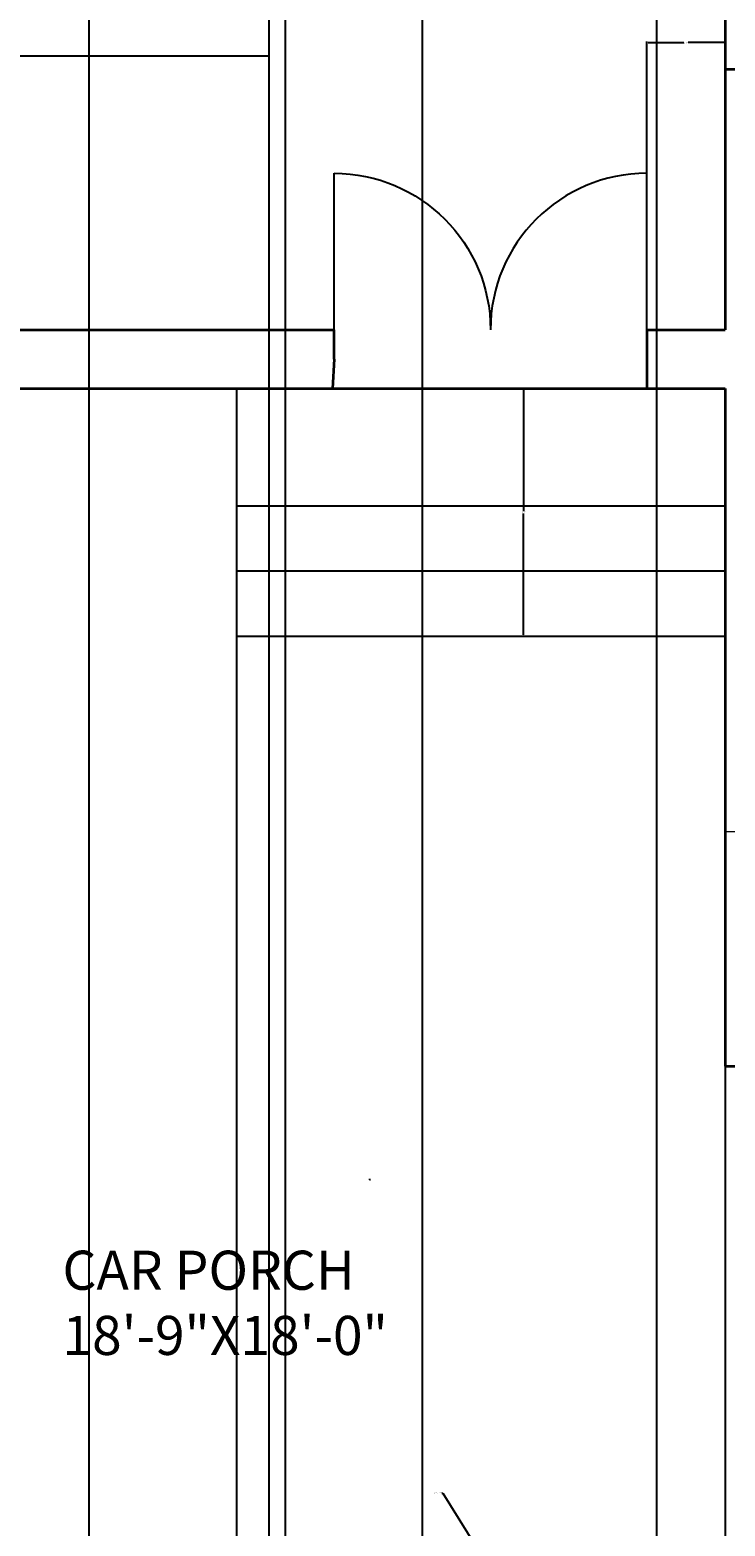
# Model space of a CAD drawing. Units: inches. Extents: x -10 to 502, y -868 to 56.
# Tile 7 of 14: x 165 to 272, y -724 to -495. Entities that reach past the tile are written whole.
import ezdxf

# ---------------------------------------------------------------- set-up
doc = ezdxf.new("R2010")
doc.units = ezdxf.units.IN
doc.header["$MEASUREMENT"] = 0
for name, color, linetype, lineweight in [('A-ANNO-DIMS', 2, 'Continuous', 18), ('A-AREA-IDEN', 7, 'Continuous', 18), ('A-DOOR', 4, 'Continuous', 25), ('A-FLOR-STRS', 7, 'Continuous', 25), ('A-GLAZ', 162, 'Continuous', 18), ('A-WALL', 7, 'Continuous', 35)]:
    doc.layers.add(name, color=color, linetype=linetype, lineweight=lineweight)
doc.styles.get("Standard").update_dxf_attribs({"font": 'arial.ttf'})
doc.dimstyles.get("Standard").update_dxf_attribs({"dimtxt": 0.18, "dimasz": 0.18, "dimexe": 0.18, "dimexo": 0.0625, "dimgap": 0.09, "dimtad": 0, "dimtih": 1, "dimtoh": 1, "dimdec": 0, "dimzin": 0, "dimdsep": 46, "dimlunit": 3, "dimtxsty": 'Standard', "dimcen": 0.09, "dimadec": 0, "dimazin": 0, "dimtfac": 1, "dimtdec": 0, "dimtofl": 0, "dimtmove": 0, "dimatfit": 3, "dimfxl": 1, "dimtolj": 1, "dimtzin": 0, "dimarcsym": 0})

# ---------------------------------------------------------------- blocks, each defined once
blk = doc.blocks.new('DOOR-SWING-24IN')
blk.add_line((24, 0), (24, 24))
blk.add_arc((24, 0), 24, 90, 180)
blk = doc.blocks.new('*D45')
at = {"layer": 'A-ANNO-DIMS', "color": 0, "lineweight": -2, "transparency": 16777216}
for p, q in [((196.98, -587.92), (196.98, -846.58)), ((271.95, -587.92), (271.95, -846.58)), ((197.16, -846.4), (234.14, -846.4)), ((271.77, -846.4), (234.8, -846.4))]:
    blk.add_line(p, q, dxfattribs=at)
at = {"layer": 'A-ANNO-DIMS', "color": 0, "transparency": 16777216}
for points in [[(197.16, -846.37), (197.16, -846.43), (196.98, -846.4)], [(271.77, -846.37), (271.77, -846.43), (271.95, -846.4)]]:
    blk.add_solid(points, dxfattribs=at)
at = {"layer": 'Defpoints', "color": 0, "transparency": 16777216}
for p in [(196.98, -587.85), (271.95, -587.85), (271.95, -846.4)]:
    blk.add_point(p, dxfattribs=at)
at = {"layer": 'A-ANNO-DIMS', "color": 0, "transparency": 16777216, "insert": (234.47, -846.4), "char_height": 0.18, "attachment_point": 5}
blk.add_mtext('\\A1;6\'-3"', dxfattribs=at)
blk = doc.blocks.new('*D46')
at = {"layer": 'A-ANNO-DIMS', "color": 0, "lineweight": -2, "transparency": 16777216}
for p, q in [((197.04, -549.85), (241.21, -549.85)), ((241.03, -550.03), (241.03, -568.67)), ((241.03, -587.67), (241.03, -569.03)), ((197.04, -587.85), (241.21, -587.85))]:
    blk.add_line(p, q, dxfattribs=at)
at = {"layer": 'A-ANNO-DIMS', "color": 0, "transparency": 16777216}
for points in [[(241, -550.03), (241.06, -550.03), (241.03, -549.85)], [(241, -587.67), (241.06, -587.67), (241.03, -587.85)]]:
    blk.add_solid(points, dxfattribs=at)
at = {"layer": 'Defpoints', "color": 0, "transparency": 16777216}
for p in [(196.98, -549.85), (196.98, -587.85), (241.03, -587.85)]:
    blk.add_point(p, dxfattribs=at)
at = {"layer": 'A-ANNO-DIMS', "color": 0, "transparency": 16777216, "insert": (241.03, -568.85), "char_height": 0.18, "attachment_point": 5}
blk.add_mtext('\\A1;3\'-2"', dxfattribs=at)
blk = doc.blocks.new('*D47')
at = {"layer": 'A-ANNO-DIMS', "color": 0, "lineweight": -2, "transparency": 16777216}
for p, q in [((91.95, -494.92), (91.95, -846.58)), ((201.95, -494.92), (201.95, -846.58)), ((92.13, -846.4), (146.62, -846.4)), ((201.77, -846.4), (147.28, -846.4))]:
    blk.add_line(p, q, dxfattribs=at)
at = {"layer": 'A-ANNO-DIMS', "color": 0, "transparency": 16777216}
for points in [[(92.13, -846.37), (92.13, -846.43), (91.95, -846.4)], [(201.77, -846.37), (201.77, -846.43), (201.95, -846.4)]]:
    blk.add_solid(points, dxfattribs=at)
at = {"layer": 'Defpoints', "color": 0, "transparency": 16777216}
for p in [(91.95, -494.85), (201.95, -494.85), (201.95, -846.4)]:
    blk.add_point(p, dxfattribs=at)
at = {"layer": 'A-ANNO-DIMS', "color": 0, "transparency": 16777216, "insert": (146.95, -846.4), "char_height": 0.18, "attachment_point": 5}
blk.add_mtext('\\A1;9\'-2"', dxfattribs=at)
blk = doc.blocks.new('*D53')
at = {"layer": 'A-ANNO-DIMS', "color": 0, "lineweight": -2, "transparency": 16777216}
for p, q in [((174.32, -443.06), (174.32, -846.58)), ((204.45, -443.92), (204.45, -846.58)), ((174.5, -846.4), (189.05, -846.4)), ((204.27, -846.4), (189.72, -846.4))]:
    blk.add_line(p, q, dxfattribs=at)
at = {"layer": 'A-ANNO-DIMS', "color": 0, "transparency": 16777216}
for points in [[(174.5, -846.37), (174.5, -846.43), (174.32, -846.4)], [(204.27, -846.37), (204.27, -846.43), (204.45, -846.4)]]:
    blk.add_solid(points, dxfattribs=at)
at = {"layer": 'Defpoints', "color": 0, "transparency": 16777216}
for p in [(174.32, -443), (204.45, -443.85), (204.45, -846.4)]:
    blk.add_point(p, dxfattribs=at)
at = {"layer": 'A-ANNO-DIMS', "color": 0, "transparency": 16777216, "insert": (189.39, -846.4), "char_height": 0.18, "attachment_point": 5}
blk.add_mtext('\\A1;2\'-6"', dxfattribs=at)
blk = doc.blocks.new('*D57')
at = {"layer": 'A-ANNO-DIMS', "color": 0, "lineweight": -2, "transparency": 16777216}
for p, q in [((259.95, -540.79), (259.95, -496.62)), ((260.13, -496.8), (265.63, -496.8)), ((271.77, -496.8), (266.27, -496.8)), ((271.95, -540.79), (271.95, -496.62))]:
    blk.add_line(p, q, dxfattribs=at)
at = {"layer": 'A-ANNO-DIMS', "color": 0, "transparency": 16777216}
for points in [[(260.13, -496.77), (260.13, -496.83), (259.95, -496.8)], [(271.77, -496.77), (271.77, -496.83), (271.95, -496.8)]]:
    blk.add_solid(points, dxfattribs=at)
at = {"layer": 'Defpoints', "color": 0, "transparency": 16777216}
for p in [(271.95, -496.8), (259.95, -540.85), (271.95, -540.85)]:
    blk.add_point(p, dxfattribs=at)
at = {"layer": 'A-ANNO-DIMS', "color": 0, "transparency": 16777216, "insert": (265.95, -496.8), "char_height": 0.18, "attachment_point": 5}
blk.add_mtext('\\A1;1\'-0"', dxfattribs=at)
blk = doc.blocks.new('*D65')
at = {"layer": 'A-ANNO-DIMS', "color": 0, "lineweight": -2, "transparency": 16777216}
for p, q in [((225.45, -263.92), (225.45, -846.58)), ((261.45, -263.92), (261.45, -846.58)), ((225.63, -846.4), (243.12, -846.4)), ((261.27, -846.4), (243.78, -846.4))]:
    blk.add_line(p, q, dxfattribs=at)
at = {"layer": 'A-ANNO-DIMS', "color": 0, "transparency": 16777216}
for points in [[(225.63, -846.37), (225.63, -846.43), (225.45, -846.4)], [(261.27, -846.37), (261.27, -846.43), (261.45, -846.4)]]:
    blk.add_solid(points, dxfattribs=at)
at = {"layer": 'Defpoints', "color": 0, "transparency": 16777216}
for p in [(225.45, -263.85), (261.45, -263.85), (261.45, -846.4)]:
    blk.add_point(p, dxfattribs=at)
at = {"layer": 'A-ANNO-DIMS', "color": 0, "transparency": 16777216, "insert": (243.45, -846.4), "char_height": 0.18, "attachment_point": 5}
blk.add_mtext('\\A1;3\'-0"', dxfattribs=at)
blk = doc.blocks.new('*D66')
at = {"layer": 'A-ANNO-DIMS', "color": 0, "lineweight": -2, "transparency": 16777216}
for p, q in [((217.36, -671.21), (217.54, -671.21)), ((217.45, -671.3), (217.45, -671.12)), ((144.25, -867.86), (171.64, -794.28)), ((144.07, -867.86), (144.25, -867.86))]:
    blk.add_line(p, q, dxfattribs=at)
at = {"layer": 'A-ANNO-DIMS', "color": 0, "transparency": 16777216}
blk.add_solid([(171.61, -794.27), (171.67, -794.29), (171.7, -794.11)], dxfattribs=at)
at = {"layer": 'Defpoints', "color": 0, "transparency": 16777216}
for p in [(217.45, -671.21), (171.7, -794.11)]:
    blk.add_point(p, dxfattribs=at)
at = {"layer": 'A-ANNO-DIMS', "color": 0, "transparency": 16777216, "insert": (143.32, -867.86), "char_height": 0.18, "attachment_point": 5}
blk.add_mtext('\\A1;2X R10\'-11"', dxfattribs=at)
blk = doc.blocks.new('*D67')
at = {"layer": 'A-ANNO-DIMS', "color": 0, "lineweight": -2, "transparency": 16777216}
for p, q in [((228.48, -719.35), (228.66, -719.35)), ((228.66, -719.35), (244.8, -745.4)), ((271.86, -789.23), (272.04, -789.23)), ((271.95, -789.32), (271.95, -789.14))]:
    blk.add_line(p, q, dxfattribs=at)
at = {"layer": 'A-ANNO-DIMS', "color": 0, "transparency": 16777216}
blk.add_solid([(244.82, -745.39), (244.77, -745.42), (244.89, -745.56)], dxfattribs=at)
at = {"layer": 'Defpoints', "color": 0, "transparency": 16777216}
for p in [(244.89, -745.56), (271.95, -789.23)]:
    blk.add_point(p, dxfattribs=at)
at = {"layer": 'A-ANNO-DIMS', "color": 0, "transparency": 16777216, "insert": (227.85, -719.35), "char_height": 0.18, "attachment_point": 5}
blk.add_mtext('\\A1;R4\'-3 1/2"', dxfattribs=at)

msp = doc.modelspace()

# ---------------------------------------------------------------- linework, layer by layer
at = {"layer": 'A-FLOR-STRS'}
for p, q in [((201.95, -452.85), (201.95, -498.85)), ((91.95, -498.85), (201.95, -498.85)), ((196.98, -549.85), (196.98, -567.85)), ((196.98, -567.85), (196.98, -577.85)), ((196.98, -567.85), (271.95, -567.85)), ((196.98, -577.85), (196.98, -587.85)), ((196.98, -577.85), (271.95, -577.85)), ((196.98, -587.85), (271.95, -587.85))]:
    msp.add_line(p, q, dxfattribs=at)
at = {"layer": 'A-GLAZ'}
for p, q in [((271.95, -617.85), (271.95, -653.85)), ((271.95, -617.85), (280.95, -617.85)), ((271.95, -653.85), (307.95, -653.85))]:
    msp.add_line(p, q, dxfattribs=at)
at = {"layer": 'A-WALL'}
for p, q in [((271.95, -452.85), (271.95, -540.85)), ((271.95, -500.85), (280.95, -500.85)), ((43.95, -540.85), (211.95, -540.85)), ((211.95, -545.35), (211.95, -540.85)), ((259.95, -540.85), (259.95, -549.85)), ((259.95, -540.85), (271.95, -540.85)), ((211.95, -545.35), (211.7, -549.85)), ((43.95, -549.85), (271.95, -549.85)), ((271.95, -549.85), (271.95, -653.85)), ((271.95, -653.85), (457.95, -653.85))]:
    msp.add_line(p, q, dxfattribs=at)

# ---------------------------------------------------------------- block references
at = {"layer": 'A-DOOR', "extrusion": (0, 0, -1), "zscale": -1}
msp.add_blockref('DOOR-SWING-24IN', (-235.95, -540.85), dxfattribs=at)
at = {"layer": 'A-DOOR'}
msp.add_blockref('DOOR-SWING-24IN', (235.95, -540.85), dxfattribs=at)

# ---------------------------------------------------------------- texts
at = {"layer": 'A-AREA-IDEN', "insert": (170.26, -682.15), "char_height": 6, "attachment_point": 1}
msp.add_mtext('CAR PORCH\\P18\'-9"X18\'-0"', dxfattribs=at)

# ---------------------------------------------------------------- dimensions: what is measured, and where the dimension line sits
at = {"layer": 'A-ANNO-DIMS'}
for base, p1, p2, picture, middle in [((261.45, -846.4), (225.45, -263.85), (261.45, -263.85), '*D65', (243.45, -846.4)), ((204.45, -846.4), (174.32, -443), (204.45, -443.85), '*D53', (189.39, -846.4)), ((201.95, -846.4), (91.95, -494.85), (201.95, -494.85), '*D47', (146.95, -846.4)), ((271.95, -496.8), (259.95, -540.85), (271.95, -540.85), '*D57', (265.95, -496.8)), ((271.95, -846.4), (196.98, -587.85), (271.95, -587.85), '*D45', (234.47, -846.4))]:
    dim = msp.add_linear_dim(base=base, p1=p1, p2=p2, dimstyle='Standard', override={"dimdec": 1, "dimlfac": 1, "dimrnd": 0, "dimzin": 1, "dimdsep": 46, "dimlunit": 4, "dimfrac": 2}, dxfattribs=at)
    dim.commit()
    dim.dimension.update_dxf_attribs({"geometry": picture, "text_midpoint": middle})
dim = msp.add_linear_dim(base=(241.03, -587.85), p1=(196.98, -549.85), p2=(196.98, -587.85), angle=270, dimstyle='Standard', override={"dimdec": 1, "dimlfac": 1, "dimrnd": 0, "dimzin": 1, "dimdsep": 46, "dimlunit": 4, "dimfrac": 2}, dxfattribs=at)
dim.commit()
dim.dimension.update_dxf_attribs({"geometry": '*D46', "text_midpoint": (241.03, -568.85)})
dim = msp.add_radius_dim(center=(217.45, -671.21), mpoint=(171.7, -794.11), text='2X <>', dimstyle='Standard', override={"dimdec": 1, "dimlfac": 1, "dimrnd": 0, "dimzin": 1, "dimdsep": 46, "dimlunit": 4, "dimfrac": 2}, dxfattribs=at)
dim.commit()
dim.dimension.update_dxf_attribs({"geometry": '*D66', "text_midpoint": (143.32, -867.86), "dimtype": 164})
dim = msp.add_radius_dim(center=(271.95, -789.23), mpoint=(244.89, -745.56), dimstyle='Standard', override={"dimdec": 1, "dimlfac": 1, "dimrnd": 0, "dimzin": 1, "dimdsep": 46, "dimlunit": 4, "dimfrac": 2}, dxfattribs=at)
dim.commit()
dim.dimension.update_dxf_attribs({"geometry": '*D67', "text_midpoint": (227.85, -719.35), "dimtype": 164})

doc.saveas('drawing.dxf')
